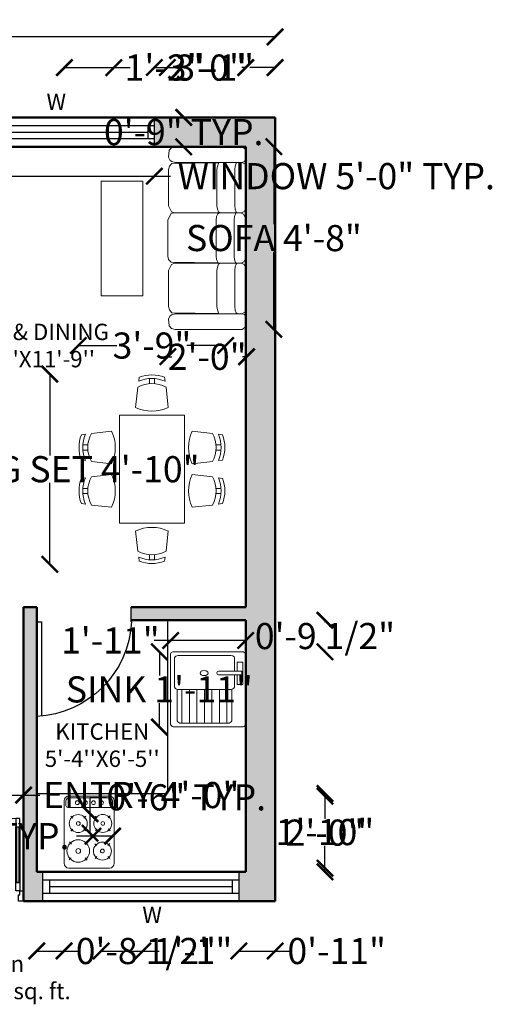
# Model space of a CAD drawing. Units: inches. Extents: x 2015 to 2400, y 1855 to 2156.
# Tile 3 of 3: x 2255 to 2400, y 1855 to 2156. Entities that reach past the tile are written whole.
import ezdxf

# ---------------------------------------------------------------- set-up
doc = ezdxf.new("R2010")
doc.units = ezdxf.units.IN
for name, color, linetype, lineweight in [('A-ANNO-DIMS', 2, 'Continuous', 18), ('A-ANNO-TEXT', 7, 'Continuous', 25), ('A-AREA-IDEN', 7, 'Continuous', 25), ('A-EQPM', 8, 'Continuous', 18), ('A-FLOR-FIXT', 9, 'Continuous', 18), ('A-FURN', 8, 'Continuous', 18), ('A-WALL-PATT', 30, 'Continuous', 13), ('Door', 40, 'Continuous', 25), ('Kitchen', 64, 'Continuous', 25), ('Walls', 7, 'Continuous', 50), ('Windows', 150, 'Continuous', 25)]:
    doc.layers.add(name, color=color, linetype=linetype, lineweight=lineweight)
doc.layers.add('A-Glaz', color=92, linetype='Continuous')
doc.styles.get("Standard").update_dxf_attribs({"font": 'arial.ttf'})
doc.dimstyles.get("Standard").update_dxf_attribs({"dimtxt": 8, "dimasz": 5, "dimexe": 0.18, "dimexo": 0.0625, "dimgap": 0.09, "dimtad": 0, "dimtih": 1, "dimtoh": 1, "dimdec": 1, "dimzin": 0, "dimdsep": 46, "dimlunit": 4, "dimtxsty": 'Standard', "dimblk": 'ARCHTICK', "dimcen": 0.09, "dimse1": 1, "dimse2": 1, "dimadec": 0, "dimazin": 0, "dimtfac": 1, "dimtdec": 1, "dimtofl": 0, "dimtmove": 0, "dimatfit": 3, "dimfxl": 1, "dimtolj": 1, "dimtzin": 0, "dimarcsym": 0})

# ---------------------------------------------------------------- blocks, each defined once
blk = doc.blocks.new('A$C13CE0A17')
at = {"layer": 'A-Glaz'}
for p, q in [((0.01, 0.61), (0.01, 0.08)), ((0.03, 0.08), (0.03, 0.61))]:
    blk.add_line(p, q, dxfattribs=at)
blk.add_lwpolyline([(1.4, 0.08), (1.4, 0.61), (1.42, 0.61), (1.42, 0.08)], close=True, dxfattribs=at)
at = {"layer": 'Door'}
for p, q in [((0, 0.61), (0, 0.69)), ((0, 0.69), (0.04, 0.69)), ((0.04, 0.69), (0.04, 0.61)), ((0, 0.61), (0, 0.08)), ((0.04, 0.61), (0, 0.61)), ((0.04, 0.61), (0, 0.61)), ((0.03, 0.61), (0.01, 0.61)), ((0.04, 0.08), (0.04, 0.61)), ((-0.035, 0), (-0.035, -0.1)), ((0, 0), (-0.035, 0)), ((0, 0.08), (0, 0)), ((0.04, 0.08), (0, 0.08)), ((0, 0.08), (0.04, 0.08)), ((0, 0), (0.04, 0)), ((0, -0.04), (0, 0)), ((0.01, 0.08), (0.03, 0.08)), ((0.04, 0), (0.04, 0.08)), ((0.015, -0.04), (0, -0.04)), ((0.015, -0.05), (0.015, -0.04)), ((0.015, -0.1), (0.015, -0.05)), ((-0.035, -0.1), (0.015, -0.1))]:
    blk.add_line(p, q, dxfattribs=at)
for points in [[(1.39, 0.69), (1.39, 0.61), (1.43, 0.61), (1.43, 0.69)], [(1.39, 0.08), (1.39, 0.61), (1.43, 0.61), (1.43, 0.08)], [(1.39, 0), (1.39, 0.08), (1.43, 0.08), (1.43, 0)], [(1.43, 0), (1.465, 0), (1.465, -0.1), (1.415, -0.1), (1.415, -0.05), (1.415, -0.04), (1.43, -0.04)]]:
    blk.add_lwpolyline(points, close=True, dxfattribs=at)
blk.add_arc((1.3872, 0.017), 0.673, 89.76573, 181.44381, dxfattribs=at)
blk.add_ellipse((0.0389, 0.0511), major_axis=(0.6669, -0.1217), ratio=0.940794, start_param=0.11153, end_param=1.73917, dxfattribs=at)
blk = doc.blocks.new('table-23')
at = {"color": 0, "linetype": 'ByBlock'}
for p, q in [((-0.632, 0.469), (-0.624, 0.525)), ((-0.485, 0.506), (-0.485, 0.436)), ((-0.415, 0.506), (-0.415, 0.436)), ((-0.268, 0.469), (-0.276, 0.525)), ((-0.675, 0.107), (-0.645, 0.387)), ((-0.225, 0.107), (-0.255, 0.387)), ((-0.9, -1.492), (-0.9, 0)), ((-0.9, 0), (0, 0)), ((0, -1.492), (0, 0)), ((-1.368, -0.264), (-1.424, -0.273)), ((-1.006, -0.221), (-1.286, -0.251)), ((0.106, -0.221), (0.386, -0.251)), ((0.468, -0.264), (0.524, -0.273)), ((-1.405, -0.411), (-1.335, -0.411)), ((-1.405, -0.481), (-1.335, -0.481)), ((0.505, -0.411), (0.435, -0.411)), ((0.505, -0.481), (0.435, -0.481)), ((-1.368, -0.628), (-1.424, -0.62)), ((-1.006, -0.671), (-1.286, -0.641)), ((0.106, -0.671), (0.386, -0.641)), ((0.468, -0.628), (0.524, -0.62)), ((-1.368, -0.864), (-1.424, -0.873)), ((-1.006, -0.821), (-1.286, -0.851)), ((0.106, -0.821), (0.386, -0.851)), ((0.468, -0.864), (0.524, -0.873)), ((-1.405, -1.011), (-1.335, -1.011)), ((-1.405, -1.081), (-1.335, -1.081)), ((0.505, -1.011), (0.435, -1.011)), ((0.505, -1.081), (0.435, -1.081)), ((-1.368, -1.228), (-1.424, -1.22)), ((0.468, -1.228), (0.524, -1.22)), ((-1.006, -1.271), (-1.286, -1.241)), ((0.106, -1.271), (0.386, -1.241)), ((-0.9, -1.492), (0, -1.492)), ((-0.675, -1.599), (-0.645, -1.879)), ((-0.225, -1.599), (-0.255, -1.879)), ((-0.632, -1.961), (-0.624, -2.017)), ((-0.485, -1.998), (-0.485, -1.928)), ((-0.415, -1.998), (-0.415, -1.928)), ((-0.268, -1.961), (-0.276, -2.017))]:
    blk.add_line(p, q, dxfattribs=at)
for centre, radius, start, end in [((-0.45, 0.077), 0.48, 68.7887, 111.2113), ((-0.45, 0.032), 0.405, 61.2372, 118.7628), ((-0.45, 0.057), 0.45, 66.1344, 113.8656), ((-0.45, 0.588), 0.531, 244.9424, 295.0576), ((-0.956, -0.446), 0.45, 156.1344, 203.8656), ((-0.931, -0.446), 0.405, 151.2372, 208.7628), ((-1.487, -0.446), 0.531, 334.9424, 25.0576), ((0.587, -0.446), 0.531, 154.9424, 205.0576), ((0.031, -0.446), 0.405, 331.2372, 28.7628), ((0.056, -0.446), 0.45, 336.1344, 23.8656), ((-0.977, -0.446), 0.48, 158.7887, 201.2113), ((0.077, -0.446), 0.48, 338.7887, 21.2113), ((-0.977, -1.046), 0.48, 158.7887, 201.2113), ((-0.956, -1.046), 0.45, 156.1344, 203.8656), ((-0.931, -1.046), 0.405, 151.2372, 208.7628), ((-1.487, -1.046), 0.531, 334.9424, 25.0576), ((0.587, -1.046), 0.531, 154.9424, 205.0576), ((0.031, -1.046), 0.405, 331.2372, 28.7628), ((0.056, -1.046), 0.45, 336.1344, 23.8656), ((0.077, -1.046), 0.48, 338.7887, 21.2113), ((-0.45, -2.081), 0.531, 64.9424, 115.0576), ((-0.45, -1.524), 0.405, 241.2372, 298.7628), ((-0.45, -1.549), 0.45, 246.1344, 293.8656), ((-0.45, -1.57), 0.48, 248.7887, 291.2113)]:
    blk.add_arc(centre, radius, start, end, dxfattribs=at)
blk = doc.blocks.new('12PCOU17')
at = {"color": 0, "linetype": 'ByBlock'}
for points in [[(-34.71, 34.72), (-33.66, 34.31), (-3.27, 34.3), (-1.81, 34.76), (-1.05, 35.2), (-0.38, 36.65), (-0.61, 39.84), (-1.73, 40.94), (-3.27, 41.4), (-33.66, 41.4), (-34.95, 40.5), (-35.65, 39.02), (-35.49, 35.83), (-34.71, 34.72)], [(-1.89, 11.91), (-1.66, 11.91), (-0.35, 14.68), (-0.35, 31.05), (-0.74, 32.58), (-1.89, 33.83), (-33.63, 34.3), (-34.84, 33.63), (-35.43, 32.38), (-35.68, 31), (-35.68, 14.74), (-35.43, 13.36), (-34.66, 11.99), (-33.44, 11.43), (-3, 11.44), (-1.66, 11.91)], [(-31.25, 11.43), (-31.06, 11.84), (-30.6, 13.09), (-30.4, 14.62), (-30.4, 31.12), (-30.6, 32.65), (-31.06, 33.9), (-31.81, 34.3)], [(-23.84, 11.43), (-22.99, 11.9), (-22.46, 13.15), (-22.23, 14.67), (-22.23, 31.07), (-22.46, 32.59), (-22.99, 33.84), (-23.12, 34.3)], [(-1.54, -10.96), (-1.31, -10.96), (0, -8.19), (0, 8.19), (-0.39, 9.71), (-1.54, 10.96), (-33.28, 11.44), (-34.5, 10.77), (-35.08, 9.51), (-35.33, 8.14), (-35.33, -8.13), (-35.08, -9.51), (-34.31, -10.87), (-33.1, -11.44), (-2.65, -11.43), (-1.31, -10.96)], [(-30.9, -11.44), (-30.72, -11.02), (-30.25, -9.77), (-30.05, -8.25), (-30.05, 8.26), (-30.25, 9.78), (-30.72, 11.03), (-31.47, 11.44)], [(-23.49, -11.44), (-22.64, -10.96), (-22.11, -9.72), (-21.88, -8.19), (-21.88, 8.2), (-22.11, 9.73), (-22.64, 10.97), (-22.77, 11.44)], [(-1.89, -11.91), (-1.66, -11.91), (-0.35, -14.68), (-0.35, -31.05), (-0.74, -32.58), (-1.89, -33.83), (-33.63, -34.3), (-34.84, -33.63), (-35.43, -32.38), (-35.68, -31), (-35.68, -14.74), (-35.43, -13.36), (-34.66, -11.99), (-33.44, -11.43), (-3, -11.44), (-1.66, -11.91)], [(-31.25, -11.43), (-31.06, -11.84), (-30.6, -13.09), (-30.4, -14.62), (-30.4, -31.12), (-30.6, -32.65), (-31.06, -33.9), (-31.81, -34.3)], [(-23.84, -11.43), (-22.99, -11.9), (-22.46, -13.15), (-22.23, -14.67), (-22.23, -31.07), (-22.46, -32.59), (-22.99, -33.84), (-23.12, -34.3)], [(-34.71, -34.72), (-33.66, -34.31), (-3.27, -34.3), (-1.81, -34.76), (-1.05, -35.2), (-0.38, -36.65), (-0.61, -39.84), (-1.73, -40.94), (-3.27, -41.4), (-33.66, -41.4), (-34.95, -40.5), (-35.65, -39.02), (-35.49, -35.83), (-34.71, -34.72)]]:
    blk.add_lwpolyline(points, dxfattribs=at)
blk = doc.blocks.new('AP0B05')
for p, q in [((35, 100), (35, 880)), ((75, 100), (75, 878.9)), ((35, 100), (35, -20)), ((815, 100), (815, -20))]:
    blk.add_line(p, q)
blk.add_lwpolyline([(35, 100), (75, 100)])
blk.add_arc((-2.4, 62.6), 818.3, 2.62122, 87.37878)
blk = doc.blocks.new('S_SINK12')
for p, q in [((0.25, 0.45), (0.25, 0)), ((0.35, 0.45), (0.35, 0)), ((0.45, 0.45), (0.45, 0)), ((0.55, 0.45), (0.55, 0)), ((0.65, 0.45), (0.65, 0)), ((0.75, 0.45), (0.75, 0)), ((0.85, 0.45), (0.85, 0))]:
    blk.add_line(p, q)
for points in [[(0, -0.469), (0, 0.469, -0.310961), (0.05, 0.5), (0.95, 0.5, -0.310466), (1, 0.469), (1, -0.469, -0.414214), (0.969, -0.5), (0.05, -0.5, -0.309971)], [(0.052, -0.195), (0.052, -0.242), (0.362, -0.242, 1), (0.362, -0.195)], [(0.5, -0.217), (0.503, -0.229, 0.107136), (0.516, -0.241, 0.076468), (0.534, -0.249), (0.554, -0.251), (0.575, -0.248, 0.076468), (0.592, -0.241, 0.107136), (0.604, -0.229), (0.608, -0.217), (0.604, -0.205, 0.107136), (0.592, -0.193, 0.076468), (0.575, -0.186), (0.554, -0.183), (0.532, -0.186, 0.076468), (0.516, -0.193, 0.107136), (0.503, -0.205)]]:
    blk.add_lwpolyline(points, format="xyb", close=True)
for points in [[(0.185, -0.001), (0.185, 0.419, -0.310466), (0.235, 0.45), (0.862, 0.45, -0.310466), (0.912, 0.419), (0.912, 0, -0.310466)], [(0.15, -0.195), (0.15, -0.031, -0.310466), (0.2, 0), (0.9, 0, -0.310466), (0.95, -0.031), (0.95, -0.419, -0.310466), (0.9, -0.45), (0.2, -0.45), (0.18, -0.448, -0.071009), (0.165, -0.442, -0.106323), (0.153, -0.432), (0.15, -0.422), (0.151, -0.419)]]:
    blk.add_lwpolyline(points, format="xyb")
for points in [[(0.114, -0.242), (0.114, -0.364), (0.039, -0.364), (0.039, -0.064), (0.114, -0.064), (0.114, -0.195)], [(0.15, -0.419), (0.15, -0.242)]]:
    blk.add_lwpolyline(points)
blk = doc.blocks.new('_ArchTick')
at = {"color": 0, "linetype": 'ByBlock', "const_width": 0.15}
blk.add_lwpolyline([(-0.5, -0.5), (0.5, 0.5)], dxfattribs=at)
blk = doc.blocks.new('*D12')
at = {"layer": 'A-ANNO-DIMS', "color": 0, "lineweight": -2, "transparency": 16777216}
for p, q in [((2093.14, 2151.23), (2206.19, 2151.23)), ((2333.14, 2151.23), (2220.09, 2151.23))]:
    blk.add_line(p, q, dxfattribs=at)
at = {"layer": 'Defpoints', "color": 0, "transparency": 16777216}
for p in [(2333.14, 2151.23), (2093.14, 2126.58), (2333.14, 2126.58)]:
    blk.add_point(p, dxfattribs=at)
at = {"layer": 'A-ANNO-DIMS', "color": 0, "lineweight": -2, "transparency": 16777216, "xscale": 5, "yscale": 5, "zscale": 5, "rotation": 180}
blk.add_blockref('_ArchTick', (2093.14, 2151.23), dxfattribs=at)
at = {"layer": 'A-ANNO-DIMS', "color": 0, "lineweight": -2, "transparency": 16777216, "xscale": 5, "yscale": 5, "zscale": 5}
blk.add_blockref('_ArchTick', (2333.14, 2151.23), dxfattribs=at)
at = {"layer": 'A-ANNO-DIMS', "color": 0, "transparency": 16777216, "insert": (2213.14, 2151.23), "char_height": 8, "attachment_point": 5}
blk.add_mtext("\\A1;20'", dxfattribs=at)
blk = doc.blocks.new('WIN-60IN')
for p, q in [((0, 6.5), (60, 6.5)), ((2, 6.5), (2, 2.5)), ((58, 6.5), (58, 2.5)), ((2, 4.5), (58, 4.5)), ((0, 2.5), (60, 2.5))]:
    blk.add_line(p, q)
blk.add_lwpolyline([(0, 9), (60, 9), (60, 0), (0, 0)], close=True)
blk = doc.blocks.new('COOKTOP-BURNER-SMALL')
for p, q in [((0.46, 5), (1.07, 4.43)), ((5, 5.05), (4.43, 4.43)), ((0.5, 0.46), (1.08, 1.07)), ((5.05, 0.5), (4.43, 1.08))]:
    blk.add_line(p, q)
blk.add_circle((2.75, 2.75), 0.58)
for start, end in [(138.017, 221.983), (48.017, 131.983), (318.017, 41.983), (228.017, 311.983)]:
    blk.add_arc((2.75, 2.75), 2.75, start, end)
blk = doc.blocks.new('*D19')
at = {"layer": 'A-ANNO-DIMS', "color": 0, "lineweight": -2, "transparency": 16777216}
for p, q in [((2236.14, 2108.58), (2296.14, 2108.58)), ((2296.14, 2108.58), (2301.14, 2108.58))]:
    blk.add_line(p, q, dxfattribs=at)
at = {"layer": 'Defpoints', "color": 0, "transparency": 16777216}
for p in [(2236.14, 2117.58), (2296.14, 2117.58), (2296.14, 2108.58)]:
    blk.add_point(p, dxfattribs=at)
at = {"layer": 'A-ANNO-DIMS', "color": 0, "lineweight": -2, "transparency": 16777216, "xscale": 5, "yscale": 5, "zscale": 5, "rotation": 180}
blk.add_blockref('_ArchTick', (2236.14, 2108.58), dxfattribs=at)
at = {"layer": 'A-ANNO-DIMS', "color": 0, "lineweight": -2, "transparency": 16777216, "xscale": 5, "yscale": 5, "zscale": 5}
blk.add_blockref('_ArchTick', (2296.14, 2108.58), dxfattribs=at)
at = {"layer": 'A-ANNO-DIMS', "color": 0, "transparency": 16777216, "insert": (2351.85, 2108.58), "char_height": 8, "attachment_point": 5}
blk.add_mtext('\\A1;WINDOW 5\'-0" TYP.', dxfattribs=at)
blk = doc.blocks.new('*D20')
at = {"layer": 'A-ANNO-DIMS', "color": 0, "lineweight": -2, "transparency": 16777216}
for p, q in [((2305.14, 2126.58), (2305.14, 2126.26)), ((2305.14, 2117.58), (2305.14, 2117.91))]:
    blk.add_line(p, q, dxfattribs=at)
at = {"layer": 'Defpoints', "color": 0, "transparency": 16777216}
for p in [(2296.14, 2126.58), (2305.14, 2126.58), (2296.14, 2117.58)]:
    blk.add_point(p, dxfattribs=at)
at = {"layer": 'A-ANNO-DIMS', "color": 0, "lineweight": -2, "transparency": 16777216, "xscale": 5, "yscale": 5, "zscale": 5}
for p, rotation in [((2305.14, 2126.58), 90), ((2305.14, 2117.58), 270)]:
    blk.add_blockref('_ArchTick', p, dxfattribs=dict(at, rotation=rotation))
at = {"layer": 'A-ANNO-DIMS', "color": 0, "transparency": 16777216, "insert": (2305.14, 2122.08), "char_height": 8, "attachment_point": 5}
blk.add_mtext('\\A1;0\'-9" TYP.', dxfattribs=at)
blk = doc.blocks.new('*D23')
at = {"layer": 'A-ANNO-DIMS', "color": 0, "lineweight": -2, "transparency": 16777216}
for p, q in [((2277.38, 1906.51), (2272.38, 1906.51)), ((2283.36, 1906.51), (2277.38, 1906.51))]:
    blk.add_line(p, q, dxfattribs=at)
at = {"layer": 'Defpoints', "color": 0, "transparency": 16777216}
for p in [(2277.38, 1907.41), (2277.38, 1906.51), (2283.36, 1907.41)]:
    blk.add_point(p, dxfattribs=at)
at = {"layer": 'A-ANNO-DIMS', "color": 0, "lineweight": -2, "transparency": 16777216, "xscale": 5, "yscale": 5, "zscale": 5}
for p, rotation in [((2277.38, 1906.51), 179.9999999999891), ((2283.36, 1906.51), 359.9999999999891)]:
    blk.add_blockref('_ArchTick', p, dxfattribs=dict(at, rotation=rotation))
at = {"layer": 'A-ANNO-DIMS', "color": 0, "transparency": 16777216, "insert": (2222.93, 1906.51), "char_height": 8, "attachment_point": 5}
blk.add_mtext('\\A1;BURNER 0\'-6" TYP.', dxfattribs=at)
blk = doc.blocks.new('*D24')
at = {"layer": 'A-ANNO-DIMS', "color": 0, "lineweight": -2, "transparency": 16777216}
for p, q in [((2276.48, 1913.38), (2276.48, 1918.38)), ((2276.48, 1918.38), (2281.48, 1918.38)), ((2276.48, 1907.41), (2276.48, 1913.38))]:
    blk.add_line(p, q, dxfattribs=at)
at = {"layer": 'Defpoints', "color": 0, "transparency": 16777216}
for p in [(2276.48, 1913.38), (2277.38, 1913.38), (2277.38, 1907.41)]:
    blk.add_point(p, dxfattribs=at)
at = {"layer": 'A-ANNO-DIMS', "color": 0, "lineweight": -2, "transparency": 16777216, "xscale": 5, "yscale": 5, "zscale": 5}
for p, rotation in [((2276.48, 1913.38), 90), ((2276.48, 1907.41), 270)]:
    blk.add_blockref('_ArchTick', p, dxfattribs=dict(at, rotation=rotation))
at = {"layer": 'A-ANNO-DIMS', "color": 0, "transparency": 16777216, "insert": (2305.95, 1918.38), "char_height": 8, "attachment_point": 5}
blk.add_mtext('\\A1;0\'-6" TYP.', dxfattribs=at)
blk = doc.blocks.new('*D25')
at = {"layer": 'A-ANNO-DIMS', "color": 0, "lineweight": -2, "transparency": 16777216}
for p, q in [((2208.14, 1919.08), (2256.14, 1919.08)), ((2256.14, 1919.08), (2261.14, 1919.08))]:
    blk.add_line(p, q, dxfattribs=at)
at = {"layer": 'Defpoints', "color": 0, "transparency": 16777216}
for p in [(2256.14, 1919.08), (2208.14, 1911.88), (2256.14, 1911.88)]:
    blk.add_point(p, dxfattribs=at)
at = {"layer": 'A-ANNO-DIMS', "color": 0, "lineweight": -2, "transparency": 16777216, "xscale": 5, "yscale": 5, "zscale": 5, "rotation": 180}
blk.add_blockref('_ArchTick', (2208.14, 1919.08), dxfattribs=at)
at = {"layer": 'A-ANNO-DIMS', "color": 0, "lineweight": -2, "transparency": 16777216, "xscale": 5, "yscale": 5, "zscale": 5}
blk.add_blockref('_ArchTick', (2256.14, 1919.08), dxfattribs=at)
at = {"layer": 'A-ANNO-DIMS', "color": 0, "transparency": 16777216, "insert": (2292.14, 1919.08), "char_height": 8, "attachment_point": 5}
blk.add_mtext('\\A1;ENTRY 4\'-0"', dxfattribs=at)
blk = doc.blocks.new('*D27')
at = {"layer": 'A-ANNO-DIMS', "color": 0, "lineweight": -2, "transparency": 16777216}
for p, q in [((2264.14, 2047.98), (2264.14, 2023.08)), ((2264.14, 1989.73), (2264.14, 2014.63))]:
    blk.add_line(p, q, dxfattribs=at)
at = {"layer": 'Defpoints', "color": 0, "transparency": 16777216}
for p in [(2264.14, 2047.98), (2272.88, 2047.98), (2272.88, 1989.73)]:
    blk.add_point(p, dxfattribs=at)
at = {"layer": 'A-ANNO-DIMS', "color": 0, "lineweight": -2, "transparency": 16777216, "xscale": 5, "yscale": 5, "zscale": 5}
for p, rotation in [((2264.14, 2047.98), 90), ((2264.14, 1989.73), 270)]:
    blk.add_blockref('_ArchTick', p, dxfattribs=dict(at, rotation=rotation))
at = {"layer": 'A-ANNO-DIMS', "color": 0, "transparency": 16777216, "insert": (2264.14, 2018.85), "char_height": 8, "attachment_point": 5}
blk.add_mtext('\\A1;DINING SET 4\'-10"', dxfattribs=at)
blk = doc.blocks.new('*D28')
at = {"layer": 'A-ANNO-DIMS', "color": 0, "lineweight": -2, "transparency": 16777216}
for p, q in [((2272.88, 2056.71), (2284.7, 2056.71)), ((2317.96, 2056.71), (2306.14, 2056.71))]:
    blk.add_line(p, q, dxfattribs=at)
at = {"layer": 'Defpoints', "color": 0, "transparency": 16777216}
for p in [(2317.96, 2056.71), (2272.88, 2047.98), (2317.96, 2047.98)]:
    blk.add_point(p, dxfattribs=at)
at = {"layer": 'A-ANNO-DIMS', "color": 0, "lineweight": -2, "transparency": 16777216, "xscale": 5, "yscale": 5, "zscale": 5, "rotation": 180}
blk.add_blockref('_ArchTick', (2272.88, 2056.71), dxfattribs=at)
at = {"layer": 'A-ANNO-DIMS', "color": 0, "lineweight": -2, "transparency": 16777216, "xscale": 5, "yscale": 5, "zscale": 5}
blk.add_blockref('_ArchTick', (2317.96, 2056.71), dxfattribs=at)
at = {"layer": 'A-ANNO-DIMS', "color": 0, "transparency": 16777216, "insert": (2295.42, 2056.71), "char_height": 8, "attachment_point": 5}
blk.add_mtext('\\A1;3\'-9"', dxfattribs=at)
blk = doc.blocks.new('*D29')
at = {"layer": 'A-ANNO-DIMS', "color": 0, "lineweight": -2, "transparency": 16777216}
for p, q in [((2332.76, 2117.58), (2332.76, 2093.85)), ((2332.76, 2061.66), (2332.76, 2085.39))]:
    blk.add_line(p, q, dxfattribs=at)
at = {"layer": 'Defpoints', "color": 0, "transparency": 16777216}
for p in [(2324.37, 2117.58), (2324.37, 2061.66), (2332.76, 2061.66)]:
    blk.add_point(p, dxfattribs=at)
at = {"layer": 'A-ANNO-DIMS', "color": 0, "lineweight": -2, "transparency": 16777216, "xscale": 5, "yscale": 5, "zscale": 5}
for p, rotation in [((2332.76, 2117.58), 90), ((2332.76, 2061.66), 270)]:
    blk.add_blockref('_ArchTick', p, dxfattribs=dict(at, rotation=rotation))
at = {"layer": 'A-ANNO-DIMS', "color": 0, "transparency": 16777216, "insert": (2332.76, 2089.62), "char_height": 8, "attachment_point": 5}
blk.add_mtext('\\A1;SOFA 4\'-8"', dxfattribs=at)
blk = doc.blocks.new('*D30')
at = {"layer": 'A-ANNO-DIMS', "color": 0, "lineweight": -2, "transparency": 16777216}
for p, q in [((2300.28, 2053.27), (2301.53, 2053.27)), ((2324.37, 2053.27), (2323.12, 2053.27))]:
    blk.add_line(p, q, dxfattribs=at)
at = {"layer": 'Defpoints', "color": 0, "transparency": 16777216}
for p in [(2300.28, 2061.66), (2324.37, 2061.66), (2300.28, 2053.27)]:
    blk.add_point(p, dxfattribs=at)
at = {"layer": 'A-ANNO-DIMS', "color": 0, "lineweight": -2, "transparency": 16777216, "xscale": 5, "yscale": 5, "zscale": 5, "rotation": 180}
blk.add_blockref('_ArchTick', (2300.28, 2053.27), dxfattribs=at)
at = {"layer": 'A-ANNO-DIMS', "color": 0, "lineweight": -2, "transparency": 16777216, "xscale": 5, "yscale": 5, "zscale": 5}
blk.add_blockref('_ArchTick', (2324.37, 2053.27), dxfattribs=at)
at = {"layer": 'A-ANNO-DIMS', "color": 0, "transparency": 16777216, "insert": (2312.33, 2053.27), "char_height": 8, "attachment_point": 5}
blk.add_mtext('\\A1;2\'-0"', dxfattribs=at)
blk = doc.blocks.new('*D35')
at = {"layer": 'A-ANNO-DIMS', "color": 0, "lineweight": -2, "transparency": 16777216}
for p, q in [((2297.69, 1962.95), (2297.69, 1955.66)), ((2297.69, 1939.91), (2297.69, 1947.21))]:
    blk.add_line(p, q, dxfattribs=at)
at = {"layer": 'Defpoints', "color": 0, "transparency": 16777216}
for p in [(2301.14, 1962.95), (2297.69, 1939.91), (2301.14, 1939.91)]:
    blk.add_point(p, dxfattribs=at)
at = {"layer": 'A-ANNO-DIMS', "color": 0, "lineweight": -2, "transparency": 16777216, "xscale": 5, "yscale": 5, "zscale": 5}
for p, rotation in [((2297.69, 1962.95), 90), ((2297.69, 1939.91), 270)]:
    blk.add_blockref('_ArchTick', p, dxfattribs=dict(at, rotation=rotation))
at = {"layer": 'A-ANNO-DIMS', "color": 0, "transparency": 16777216, "insert": (2297.69, 1951.43), "char_height": 8, "attachment_point": 5}
blk.add_mtext('\\A1;SINK 1\'-11"', dxfattribs=at)
blk = doc.blocks.new('*D36')
at = {"layer": 'A-ANNO-DIMS', "color": 0, "lineweight": -2, "transparency": 16777216}
for p, q in [((2301.14, 1966.41), (2296.14, 1966.41)), ((2324.14, 1966.41), (2301.14, 1966.41))]:
    blk.add_line(p, q, dxfattribs=at)
at = {"layer": 'Defpoints', "color": 0, "transparency": 16777216}
for p in [(2301.14, 1966.41), (2301.14, 1962.95), (2324.14, 1962.95)]:
    blk.add_point(p, dxfattribs=at)
at = {"layer": 'A-ANNO-DIMS', "color": 0, "lineweight": -2, "transparency": 16777216, "xscale": 5, "yscale": 5, "zscale": 5, "rotation": 180}
blk.add_blockref('_ArchTick', (2301.14, 1966.41), dxfattribs=at)
at = {"layer": 'A-ANNO-DIMS', "color": 0, "lineweight": -2, "transparency": 16777216, "xscale": 5, "yscale": 5, "zscale": 5}
blk.add_blockref('_ArchTick', (2324.14, 1966.41), dxfattribs=at)
at = {"layer": 'A-ANNO-DIMS', "color": 0, "transparency": 16777216, "insert": (2282.69, 1966.41), "char_height": 8, "attachment_point": 5}
blk.add_mtext('\\A1;1\'-11"', dxfattribs=at)
blk = doc.blocks.new('*D38')
at = {"layer": 'A-ANNO-DIMS', "color": 0, "lineweight": -2, "transparency": 16777216}
for p, q in [((2322.02, 1871.33), (2333.14, 1871.33)), ((2333.14, 1871.33), (2338.14, 1871.33))]:
    blk.add_line(p, q, dxfattribs=at)
at = {"layer": 'Defpoints', "color": 0, "transparency": 16777216}
for p in [(2322.02, 1886.58), (2333.14, 1886.58), (2333.14, 1871.33)]:
    blk.add_point(p, dxfattribs=at)
at = {"layer": 'A-ANNO-DIMS', "color": 0, "lineweight": -2, "transparency": 16777216, "xscale": 5, "yscale": 5, "zscale": 5, "rotation": 180}
blk.add_blockref('_ArchTick', (2322.02, 1871.33), dxfattribs=at)
at = {"layer": 'A-ANNO-DIMS', "color": 0, "lineweight": -2, "transparency": 16777216, "xscale": 5, "yscale": 5, "zscale": 5}
blk.add_blockref('_ArchTick', (2333.14, 1871.33), dxfattribs=at)
at = {"layer": 'A-ANNO-DIMS', "color": 0, "transparency": 16777216, "insert": (2351.97, 1871.33), "char_height": 8, "attachment_point": 5}
blk.add_mtext('\\A1;0\'-11"', dxfattribs=at)
blk = doc.blocks.new('*D39')
at = {"layer": 'A-ANNO-DIMS', "color": 0, "lineweight": -2, "transparency": 16777216}
for p, q in [((2296.14, 2141.83), (2303.92, 2141.83)), ((2333.14, 2141.83), (2325.36, 2141.83))]:
    blk.add_line(p, q, dxfattribs=at)
at = {"layer": 'Defpoints', "color": 0, "transparency": 16777216}
for p in [(2333.14, 2141.83), (2296.14, 2126.58), (2333.14, 2126.58)]:
    blk.add_point(p, dxfattribs=at)
at = {"layer": 'A-ANNO-DIMS', "color": 0, "lineweight": -2, "transparency": 16777216, "xscale": 5, "yscale": 5, "zscale": 5, "rotation": 180}
blk.add_blockref('_ArchTick', (2296.14, 2141.83), dxfattribs=at)
at = {"layer": 'A-ANNO-DIMS', "color": 0, "lineweight": -2, "transparency": 16777216, "xscale": 5, "yscale": 5, "zscale": 5}
blk.add_blockref('_ArchTick', (2333.14, 2141.83), dxfattribs=at)
at = {"layer": 'A-ANNO-DIMS', "color": 0, "transparency": 16777216, "insert": (2314.64, 2141.83), "char_height": 8, "attachment_point": 5}
blk.add_mtext('\\A1;3\'-1"', dxfattribs=at)
blk = doc.blocks.new('*D45')
at = {"layer": 'A-ANNO-DIMS', "color": 0, "lineweight": -2, "transparency": 16777216}
for p, q in [((2348.39, 1919.58), (2348.39, 1911.76)), ((2348.39, 1895.58), (2348.39, 1903.41))]:
    blk.add_line(p, q, dxfattribs=at)
at = {"layer": 'Defpoints', "color": 0, "transparency": 16777216}
for p in [(2300.14, 1919.58), (2324.14, 1895.58), (2348.39, 1895.58)]:
    blk.add_point(p, dxfattribs=at)
at = {"layer": 'A-ANNO-DIMS', "color": 0, "lineweight": -2, "transparency": 16777216, "xscale": 5, "yscale": 5, "zscale": 5}
for p, rotation in [((2348.39, 1919.58), 90), ((2348.39, 1895.58), 270)]:
    blk.add_blockref('_ArchTick', p, dxfattribs=dict(at, rotation=rotation))
at = {"layer": 'A-ANNO-DIMS', "color": 0, "transparency": 16777216, "insert": (2348.39, 1907.58), "char_height": 8, "attachment_point": 5}
blk.add_mtext('\\A1;2\'-0"', dxfattribs=at)
blk = doc.blocks.new('*D46')
at = {"layer": 'A-ANNO-DIMS', "color": 0, "lineweight": -2, "transparency": 16777216}
for p, q in [((2300.14, 2141.83), (2301.35, 2141.83)), ((2324.14, 2141.83), (2322.93, 2141.83))]:
    blk.add_line(p, q, dxfattribs=at)
at = {"layer": 'Defpoints', "color": 0, "transparency": 16777216}
for p in [(2324.14, 2141.83), (2300.14, 1972.58), (2324.14, 1972.58)]:
    blk.add_point(p, dxfattribs=at)
at = {"layer": 'A-ANNO-DIMS', "color": 0, "lineweight": -2, "transparency": 16777216, "xscale": 5, "yscale": 5, "zscale": 5, "rotation": 180}
blk.add_blockref('_ArchTick', (2300.14, 2141.83), dxfattribs=at)
at = {"layer": 'A-ANNO-DIMS', "color": 0, "lineweight": -2, "transparency": 16777216, "xscale": 5, "yscale": 5, "zscale": 5}
blk.add_blockref('_ArchTick', (2324.14, 2141.83), dxfattribs=at)
at = {"layer": 'A-ANNO-DIMS', "color": 0, "transparency": 16777216, "insert": (2312.14, 2141.83), "char_height": 8, "attachment_point": 5}
blk.add_mtext('\\A1;2\'-0"', dxfattribs=at)
blk = doc.blocks.new('*D47')
at = {"layer": 'A-ANNO-DIMS', "color": 0, "lineweight": -2, "transparency": 16777216}
for p, q in [((2348.39, 1972.58), (2348.39, 1971.98)), ((2348.39, 1962.93), (2348.39, 1963.53))]:
    blk.add_line(p, q, dxfattribs=at)
at = {"layer": 'Defpoints', "color": 0, "transparency": 16777216}
for p in [(2324.14, 1972.58), (2322.99, 1962.93), (2348.39, 1962.93)]:
    blk.add_point(p, dxfattribs=at)
at = {"layer": 'A-ANNO-DIMS', "color": 0, "lineweight": -2, "transparency": 16777216, "xscale": 5, "yscale": 5, "zscale": 5}
for p, rotation in [((2348.39, 1972.58), 90), ((2348.39, 1962.93), 270)]:
    blk.add_blockref('_ArchTick', p, dxfattribs=dict(at, rotation=rotation))
at = {"layer": 'A-ANNO-DIMS', "color": 0, "transparency": 16777216, "insert": (2348.39, 1967.76), "char_height": 8, "attachment_point": 5}
blk.add_mtext('\\A1;0\'-9 1/2"', dxfattribs=at)
blk = doc.blocks.new('*D48')
at = {"layer": 'A-ANNO-DIMS', "color": 0, "lineweight": -2, "transparency": 16777216}
for p, q in [((2260.14, 1871.33), (2268.52, 1871.33)), ((2268.52, 1871.33), (2273.52, 1871.33))]:
    blk.add_line(p, q, dxfattribs=at)
at = {"layer": 'Defpoints', "color": 0, "transparency": 16777216}
for p in [(2268.52, 1898.18), (2260.14, 1895.58), (2268.52, 1871.33)]:
    blk.add_point(p, dxfattribs=at)
at = {"layer": 'A-ANNO-DIMS', "color": 0, "lineweight": -2, "transparency": 16777216, "xscale": 5, "yscale": 5, "zscale": 5, "rotation": 180}
blk.add_blockref('_ArchTick', (2260.14, 1871.33), dxfattribs=at)
at = {"layer": 'A-ANNO-DIMS', "color": 0, "lineweight": -2, "transparency": 16777216, "xscale": 5, "yscale": 5, "zscale": 5}
blk.add_blockref('_ArchTick', (2268.52, 1871.33), dxfattribs=at)
at = {"layer": 'A-ANNO-DIMS', "color": 0, "transparency": 16777216, "insert": (2293.57, 1871.33), "char_height": 8, "attachment_point": 5}
blk.add_mtext('\\A1;0\'-8 1/2"', dxfattribs=at)
blk = doc.blocks.new('*D49')
at = {"layer": 'A-ANNO-DIMS', "color": 0, "lineweight": -2, "transparency": 16777216}
for p, q in [((2279.88, 1871.33), (2292.63, 1871.33)), ((2292.63, 1871.33), (2297.63, 1871.33))]:
    blk.add_line(p, q, dxfattribs=at)
at = {"layer": 'Defpoints', "color": 0, "transparency": 16777216}
for p in [(2279.88, 2071.97), (2292.63, 2071.97), (2292.63, 1871.33)]:
    blk.add_point(p, dxfattribs=at)
at = {"layer": 'A-ANNO-DIMS', "color": 0, "lineweight": -2, "transparency": 16777216, "xscale": 5, "yscale": 5, "zscale": 5, "rotation": 180}
blk.add_blockref('_ArchTick', (2279.88, 1871.33), dxfattribs=at)
at = {"layer": 'A-ANNO-DIMS', "color": 0, "lineweight": -2, "transparency": 16777216, "xscale": 5, "yscale": 5, "zscale": 5}
blk.add_blockref('_ArchTick', (2292.63, 1871.33), dxfattribs=at)
at = {"layer": 'A-ANNO-DIMS', "color": 0, "transparency": 16777216, "insert": (2307.98, 1871.33), "char_height": 8, "attachment_point": 5}
blk.add_mtext('\\A1;1\'-1"', dxfattribs=at)
blk = doc.blocks.new('*D50')
at = {"layer": 'A-ANNO-DIMS', "color": 0, "lineweight": -2, "transparency": 16777216}
for p, q in [((2077.89, 2107.02), (2077.89, 2093.6)), ((2077.89, 2071.97), (2077.89, 2085.39))]:
    blk.add_line(p, q, dxfattribs=at)
at = {"layer": 'Defpoints', "color": 0, "transparency": 16777216}
for p in [(2077.89, 2107.02), (2279.88, 2107.02), (2279.88, 2071.97)]:
    blk.add_point(p, dxfattribs=at)
at = {"layer": 'A-ANNO-DIMS', "color": 0, "lineweight": -2, "transparency": 16777216, "xscale": 5, "yscale": 5, "zscale": 5}
for p, rotation in [((2077.89, 2107.02), 90), ((2077.89, 2071.97), 270)]:
    blk.add_blockref('_ArchTick', p, dxfattribs=dict(at, rotation=rotation))
at = {"layer": 'A-ANNO-DIMS', "color": 0, "transparency": 16777216, "insert": (2077.89, 2089.49), "char_height": 8, "attachment_point": 5}
blk.add_mtext('\\A1;2\'-11"', dxfattribs=at)
blk = doc.blocks.new('*D51')
at = {"layer": 'A-ANNO-DIMS', "color": 0, "lineweight": -2, "transparency": 16777216}
for p, q in [((2268.64, 2141.83), (2283.77, 2141.83)), ((2283.77, 2141.83), (2288.77, 2141.83))]:
    blk.add_line(p, q, dxfattribs=at)
at = {"layer": 'Defpoints', "color": 0, "transparency": 16777216}
for p in [(2283.77, 2141.83), (2268.64, 1917.87), (2283.77, 1917.87)]:
    blk.add_point(p, dxfattribs=at)
at = {"layer": 'A-ANNO-DIMS', "color": 0, "lineweight": -2, "transparency": 16777216, "xscale": 5, "yscale": 5, "zscale": 5, "rotation": 180}
blk.add_blockref('_ArchTick', (2268.64, 2141.83), dxfattribs=at)
at = {"layer": 'A-ANNO-DIMS', "color": 0, "lineweight": -2, "transparency": 16777216, "xscale": 5, "yscale": 5, "zscale": 5}
blk.add_blockref('_ArchTick', (2283.77, 2141.83), dxfattribs=at)
at = {"layer": 'A-ANNO-DIMS', "color": 0, "transparency": 16777216, "insert": (2299.12, 2141.83), "char_height": 8, "attachment_point": 5}
blk.add_mtext('\\A1;1\'-3"', dxfattribs=at)
blk = doc.blocks.new('*D52')
at = {"layer": 'A-ANNO-DIMS', "color": 0, "lineweight": -2, "transparency": 16777216}
for p, q in [((2348.39, 1918.76), (2348.39, 1911.92)), ((2348.39, 1896.73), (2348.39, 1903.57))]:
    blk.add_line(p, q, dxfattribs=at)
at = {"layer": 'Defpoints', "color": 0, "transparency": 16777216}
for p in [(2282.44, 1918.76), (2348.39, 1918.76), (2282.44, 1896.73)]:
    blk.add_point(p, dxfattribs=at)
at = {"layer": 'A-ANNO-DIMS', "color": 0, "lineweight": -2, "transparency": 16777216, "xscale": 5, "yscale": 5, "zscale": 5}
for p, rotation in [((2348.39, 1918.76), 90), ((2348.39, 1896.73), 270)]:
    blk.add_blockref('_ArchTick', p, dxfattribs=dict(at, rotation=rotation))
at = {"layer": 'A-ANNO-DIMS', "color": 0, "transparency": 16777216, "insert": (2348.39, 1907.74), "char_height": 8, "attachment_point": 5}
blk.add_mtext('\\A1;1\'-10"', dxfattribs=at)

msp = doc.modelspace()

# ---------------------------------------------------------------- hatches: boundary and pattern name
at = {"layer": 'A-WALL-PATT'}
h = msp.add_hatch(color=256, dxfattribs=at)
h.dxf.hatch_style = 1
h.paths.add_polyline_path([(2236.14, 2126.58), (2093.14, 2126.58), (2093.14, 2111.58), (2102.14, 2111.58), (2102.14, 2111.85), (2102.14, 2117.58), (2204.14, 2117.58), (2204.14, 2005.56), (2208.14, 2005.56), (2208.14, 2117.58), (2236.14, 2117.58)])
h.paths.add_polyline_path([(2102.14, 2077.58), (2175.16, 2077.58), (2175.16, 2081.58), (2102.14, 2081.58), (2102.14, 2087.58), (2093.14, 2087.58), (2093.14, 2057.08), (2102.14, 2057.08), (2102.14, 2057.96)], flags=17)
h.paths.add_polyline_path([(2208.14, 1976.58), (2203.68, 1976.58), (2174.71, 1976.58), (2102.14, 1976.58), (2102.14, 1997.08), (2093.14, 1997.08), (2093.14, 1943.58), (2102.14, 1943.58), (2102.14, 1967.58), (2208.14, 1967.58)])
h.paths.add_polyline_path([(2260.14, 1976.58), (2256.14, 1976.58), (2256.14, 1886.58), (2262.02, 1886.58), (2262.02, 1895.58), (2260.14, 1895.58)])
h.paths.add_polyline_path([(2208.14, 1895.58), (2102.14, 1895.58), (2102.14, 1919.58), (2093.14, 1919.58), (2093.14, 1886.58), (2208.14, 1886.58)])
h = msp.add_hatch(color=256, dxfattribs=at)
h.dxf.hatch_style = 1
h.paths.add_polyline_path([(2333.14, 2126.58), (2296.14, 2126.58), (2296.14, 2117.58), (2324.14, 2117.58), (2324.14, 2116.43), (2324.35, 2115.97), (2324.24, 2113.82), (2324.14, 2113.67), (2324.14, 2111.63), (2324.21, 2111.49), (2324.37, 2110.56), (2324.37, 2098.94), (2324.14, 2098.53), (2324.14, 2080.71), (2324.21, 2080.6), (2324.37, 2079.67), (2324.37, 2068.68), (2324.14, 1976.58), (2289.11, 1976.58), (2289.11, 1972.58), (2324.14, 1972.58), (2324.14, 1895.58), (2322.02, 1895.58), (2322.02, 1886.58), (2333.14, 1886.58)])

# ---------------------------------------------------------------- linework, layer by layer
at = {"layer": 'A-EQPM'}
for p, q in [((2282.44, 1918.76), (2269.97, 1918.76)), ((2282.44, 1918.18), (2269.97, 1918.18)), ((2268.52, 1917.31), (2268.52, 1898.18)), ((2269.1, 1917.31), (2269.1, 1915.86)), ((2269.68, 1915.28), (2282.73, 1915.28)), ((2283.31, 1915.86), (2283.31, 1917.31)), ((2283.89, 1898.18), (2283.89, 1917.31)), ((2270.58, 1912.62), (2271.2, 1912.01)), ((2275.14, 1912.64), (2274.53, 1912.03)), ((2270.61, 1908.06), (2271.22, 1908.68)), ((2275.16, 1908.09), (2274.55, 1908.69)), ((2270.15, 1904.77), (2270.79, 1904.09)), ((2275.7, 1904.67), (2275.01, 1904.03)), ((2270.05, 1899.23), (2270.73, 1899.86)), ((2275.59, 1899.12), (2274.95, 1899.81)), ((2269.97, 1896.73), (2282.44, 1896.73))]:
    msp.add_line(p, q, dxfattribs=at)
for centre, radius in [((2272.58, 1916.73), 0.58), ((2275.05, 1916.73), 0.58), ((2277.51, 1916.73), 0.58), ((2279.97, 1916.73), 0.58), ((2272.87, 1910.35), 0.58), ((2272.87, 1901.95), 0.727)]:
    msp.add_circle(centre, radius, dxfattribs=at)
for centre, radius, start, end in [((2269.97, 1917.31), 1.45, 90, 180), ((2269.97, 1917.31), 0.87, 90, 180), ((2282.44, 1917.31), 1.45, 0, 90), ((2282.44, 1917.31), 0.87, 0, 90), ((2269.68, 1915.86), 0.58, 180, 270), ((2282.73, 1915.86), 0.58, 270, 0), ((2272.87, 1910.35), 2.75, 138.017, 221.983), ((2272.87, 1910.35), 2.75, 48.017, 131.983), ((2272.87, 1910.35), 2.75, 318.017, 41.983), ((2272.87, 1901.95), 3.45, 48.017, 131.983), ((2272.87, 1910.35), 2.75, 228.017, 311.983), ((2272.87, 1901.95), 3.45, 138.017, 221.983), ((2272.87, 1901.95), 3.45, 318.017, 41.983), ((2272.87, 1901.95), 3.45, 228.017, 311.983), ((2269.97, 1898.18), 1.45, 180, 270), ((2282.44, 1898.18), 1.45, 270, 0)]:
    msp.add_arc(centre, radius, start, end, dxfattribs=at)
at = {"layer": 'A-FURN'}
msp.add_lwpolyline([(2279.88, 2107.02), (2292.63, 2107.02), (2292.63, 2071.97), (2279.88, 2071.97)], close=True, dxfattribs=at)
at = {"layer": 'Kitchen'}
for p in [(2300.14, 1972.58), (2260.14, 1919.58)]:
    msp.add_line(p, (2300.14, 1919.58), dxfattribs=at)
at = {"layer": 'Walls'}
for p, q in [((2093.14, 2126.58), (2333.14, 2126.58)), ((2333.14, 2126.58), (2333.14, 1886.58)), ((2208.14, 2117.58), (2324.14, 2117.58)), ((2324.14, 2117.58), (2324.14, 1976.58)), ((2256.14, 1976.58), (2256.14, 1886.58)), ((2256.14, 1976.58), (2260.14, 1976.58)), ((2260.14, 1976.58), (2260.14, 1895.58)), ((2289.11, 1976.58), (2324.14, 1976.58)), ((2289.11, 1972.58), (2324.14, 1972.58)), ((2324.14, 1972.58), (2324.14, 1895.58)), ((2260.14, 1895.58), (2324.14, 1895.58)), ((2256.14, 1886.58), (2333.14, 1886.58))]:
    msp.add_line(p, q, dxfattribs=at)

# ---------------------------------------------------------------- block references
at = {"layer": 'A-EQPM', "rotation": 89.99999999998886}
msp.add_blockref('COOKTOP-BURNER-SMALL', (2283.12, 1907.64), dxfattribs=at)
at = {"layer": 'A-EQPM'}
msp.add_blockref('COOKTOP-BURNER-SMALL', (2277.51, 1899.19), dxfattribs=at)
at = {"layer": 'A-FLOR-FIXT', "xscale": 22.99577122507832, "yscale": 22.99577122507832, "zscale": 22.99577122507832, "rotation": 180}
msp.add_blockref('S_SINK12', (2324.14, 1951.43), dxfattribs=at)
at = {"layer": 'A-FURN', "xscale": 0.6753617326606013, "yscale": 0.6753617326606013, "zscale": 0.6753617326606013, "rotation": 180}
msp.add_blockref('12PCOU17', (2300.28, 2089.62), dxfattribs=at)
at = {"layer": 'A-FURN', "xscale": 22.16447720939163, "yscale": 22.16447720939163, "zscale": 22.16447720939163}
msp.add_blockref('table-23', (2305.39, 2035.39), dxfattribs=at)
at = {"layer": 'Door', "xscale": -0.0371474756206669, "yscale": 0.0371474756206669, "zscale": 0.0371474756206669, "rotation": 180}
msp.add_blockref('AP0B05', (2258.84, 1975.84), dxfattribs=at)
at = {"layer": 'Door', "xscale": 31.99999999999989, "yscale": 31.99999999999989, "zscale": 31.99999999999989}
msp.add_blockref('A$C13CE0A17', (2209.26, 1889.78), dxfattribs=at)
at = {"layer": 'Windows'}
for p in [(2236.14, 2117.58), (2262.02, 1886.58)]:
    msp.add_blockref('WIN-60IN', p, dxfattribs=at)

# ---------------------------------------------------------------- texts
at = {"layer": 'A-ANNO-TEXT', "char_height": 5, "attachment_point": 1}
for s, width, heights, insert in [('\\pxqc;W', 31.0576, [0], (2250.61, 2133.88)), ('\\pxqc;W', 31.0576, [0], (2279.95, 1884.9)), ('\\pxqc;Ground Floor Plan\\PBuilt Up Area : 400.00 sq. ft.', 115.2426, [17.51], (2169.7, 1869.91))]:
    msp.add_mtext_dynamic_manual_height_columns(s, width=width, gutter_width=12.5, heights=heights, dxfattribs=dict(at, insert=insert))
at = {"layer": 'A-AREA-IDEN', "char_height": 5, "attachment_point": 1}
for s, width, heights, insert in [("\\pxqc;HALL & DINING\\P9'-8''X11'-9''", 54.9856, [15.52], (2231.02, 2063.39)), ("\\pxqc;KITCHEN\\P5'-4''X6'-5''", 31.0576, [0], (2264.67, 1941.03))]:
    msp.add_mtext_dynamic_manual_height_columns(s, width=width, gutter_width=12.5, heights=heights, dxfattribs=dict(at, insert=insert))

# ---------------------------------------------------------------- dimensions: what is measured, and where the dimension line sits
at = {"layer": 'A-ANNO-DIMS'}
for base, p1, p2, override, picture, middle in [((2333.14, 2151.23), (2093.14, 2126.58), (2333.14, 2126.58), {"dimclrd": 0, "dimclre": 0, "dimclrt": 0}, '*D12', (2213.14, 2151.23)), ((2283.77, 2141.83), (2268.64, 1917.87), (2283.77, 1917.87), {"dimdec": 1, "dimlfac": 1, "dimrnd": 0, "dimzin": 1, "dimdsep": 46, "dimlunit": 4, "dimfrac": 2}, '*D51', (2299.12, 2141.83)), ((2333.14, 2141.83), (2296.14, 2126.58), (2333.14, 2126.58), {"dimdec": 1, "dimlfac": 1, "dimrnd": 0, "dimzin": 1, "dimdsep": 46, "dimlunit": 4, "dimfrac": 2}, '*D39', (2314.64, 2141.83)), ((2324.14, 2141.83), (2300.14, 1972.58), (2324.14, 1972.58), {"dimdec": 1, "dimlfac": 1, "dimrnd": 0, "dimzin": 1, "dimdsep": 46, "dimlunit": 4, "dimfrac": 2}, '*D46', (2312.14, 2141.83)), ((2292.6334, 1871.3304), (2279.8803, 2071.9679), (2292.6334, 2071.9679), {"dimdec": 1, "dimlfac": 1, "dimrnd": 0, "dimzin": 1, "dimdsep": 46, "dimlunit": 4, "dimfrac": 2}, '*D49', (2307.9799, 1871.3304)), ((2317.96, 2056.71), (2272.88, 2047.98), (2317.96, 2047.98), {"dimdec": 1, "dimlfac": 1, "dimrnd": 0, "dimzin": 1, "dimdsep": 46, "dimlunit": 4, "dimfrac": 2}, '*D28', (2295.42, 2056.71)), ((2268.52, 1871.33), (2260.14, 1895.58), (2268.52, 1898.18), {"dimdec": 1, "dimlfac": 1, "dimrnd": 0, "dimzin": 1, "dimdsep": 46, "dimlunit": 4, "dimfrac": 2}, '*D48', (2293.57, 1871.33)), ((2333.14, 1871.33), (2322.02, 1886.58), (2333.14, 1886.58), {"dimdec": 1, "dimlfac": 1, "dimrnd": 0, "dimzin": 1, "dimdsep": 46, "dimlunit": 4, "dimfrac": 2}, '*D38', (2351.97, 1871.33))]:
    dim = msp.add_linear_dim(base=base, p1=p1, p2=p2, dimstyle='Standard', override=override, dxfattribs=at)
    dim.commit()
    dim.dimension.update_dxf_attribs({"geometry": picture, "text_midpoint": middle})
for base, p1, p2, angle, text, picture, middle in [((2305.14, 2126.58), (2296.14, 2117.58), (2296.14, 2126.58), 90, '<> TYP.', '*D20', (2305.14, 2122.08)), ((2332.76, 2061.66), (2324.37, 2117.58), (2324.37, 2061.66), 270, 'SOFA <>', '*D29', (2332.76, 2089.62)), ((2264.1381, 2047.976), (2272.8755, 1989.7271), (2272.8755, 2047.976), 90, 'DINING SET <>', '*D27', (2264.1381, 2018.8516)), ((2297.69, 1939.91), (2301.14, 1962.95), (2301.14, 1939.91), 270, 'SINK <>', '*D35', (2297.69, 1951.43)), ((2276.48, 1913.38), (2277.38, 1907.41), (2277.38, 1913.38), 90, '<> TYP.', '*D24', (2305.95, 1918.38)), ((2277.38, 1906.51), (2283.36, 1907.41), (2277.38, 1907.41), 180, 'BURNER <> TYP.', '*D23', (2222.93, 1906.51))]:
    dim = msp.add_linear_dim(base=base, p1=p1, p2=p2, angle=angle, text=text, dimstyle='Standard', override={"dimdec": 1, "dimlfac": 1, "dimrnd": 0, "dimzin": 1, "dimdsep": 46, "dimlunit": 4, "dimfrac": 2}, dxfattribs=at)
    dim.commit()
    dim.dimension.update_dxf_attribs({"geometry": picture, "text_midpoint": middle})
for base, p1, p2, text, picture, middle in [((2296.14, 2108.58), (2236.14, 2117.58), (2296.14, 2117.58), 'WINDOW <> TYP.', '*D19', (2351.85, 2108.58)), ((2256.14, 1919.08), (2208.14, 1911.88), (2256.14, 1911.88), 'ENTRY <>', '*D25', (2292.14, 1919.08))]:
    dim = msp.add_linear_dim(base=base, p1=p1, p2=p2, text=text, dimstyle='Standard', override={"dimdec": 1, "dimlfac": 1, "dimrnd": 0, "dimzin": 1, "dimdsep": 46, "dimlunit": 4, "dimfrac": 2}, dxfattribs=at)
    dim.commit()
    dim.dimension.update_dxf_attribs({"geometry": picture, "text_midpoint": middle})
for base, p1, p2, angle, picture, middle in [((2077.8897, 2107.0163), (2279.8803, 2071.9679), (2279.8803, 2107.0163), 90, '*D50', (2077.8897, 2089.4921)), ((2300.28, 2053.27), (2324.37, 2061.66), (2300.28, 2061.66), 180, '*D30', (2312.33, 2053.27)), ((2348.3897, 1962.9328), (2324.1397, 1972.5804), (2322.9899, 1962.9328), 90, '*D47', (2348.3897, 1967.7566)), ((2301.14, 1966.41), (2324.14, 1962.95), (2301.14, 1962.95), 180, '*D36', (2282.69, 1966.41)), ((2348.39, 1918.76), (2282.44, 1896.73), (2282.44, 1918.76), 90, '*D52', (2348.39, 1907.74)), ((2348.39, 1895.58), (2300.14, 1919.58), (2324.14, 1895.58), 90, '*D45', (2348.39, 1907.58))]:
    dim = msp.add_linear_dim(base=base, p1=p1, p2=p2, angle=angle, dimstyle='Standard', override={"dimdec": 1, "dimlfac": 1, "dimrnd": 0, "dimzin": 1, "dimdsep": 46, "dimlunit": 4, "dimfrac": 2}, dxfattribs=at)
    dim.commit()
    dim.dimension.update_dxf_attribs({"geometry": picture, "text_midpoint": middle})

doc.saveas('drawing.dxf')
